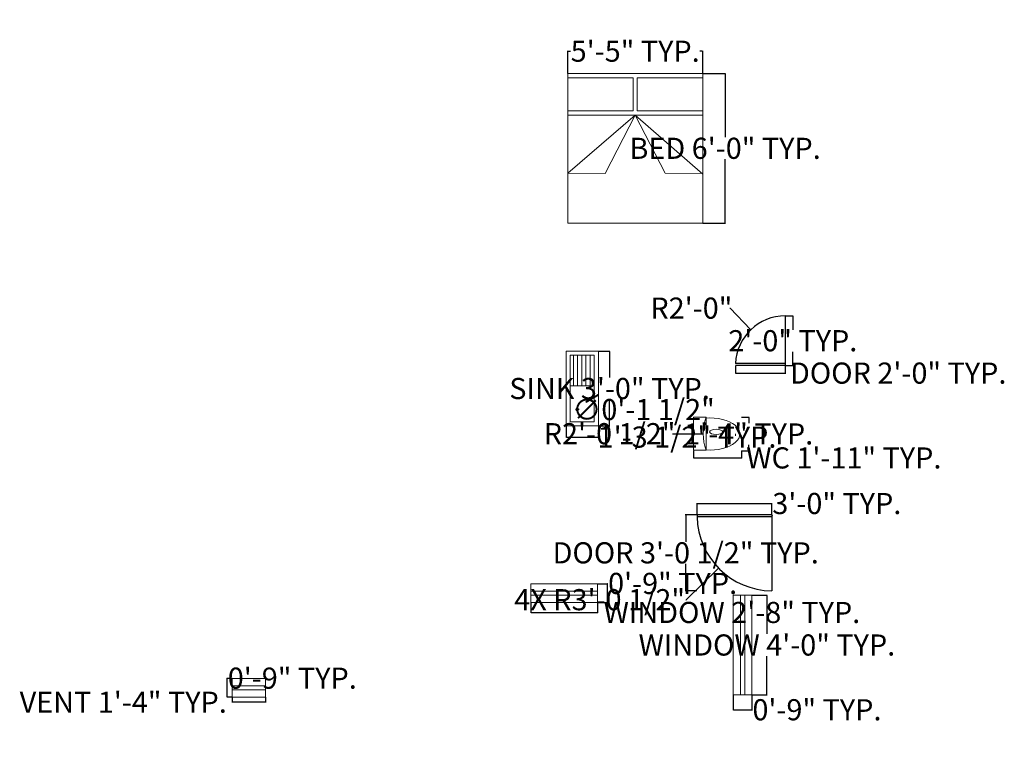
# Model space of a CAD drawing. Units: inches. Extents: x 254 to 1358, y 67 to 796.
# Tile 3 of 3: x 884 to 1358, y 443 to 796. Entities that reach past the tile are written whole.
import ezdxf

# ---------------------------------------------------------------- set-up
doc = ezdxf.new("R2010")
doc.units = ezdxf.units.IN
doc.header["$MEASUREMENT"] = 0
for name, color, linetype, lineweight in [('A-ANNO-DIMS', 2, 'Continuous', 18), ('A-FLOR-FIXT', 9, 'Continuous', 18), ('A-FURN', 8, 'Continuous', 18), ('A-GLAZ', 160, 'Continuous', 18), ('doors', 8, 'Continuous', 25)]:
    doc.layers.add(name, color=color, linetype=linetype, lineweight=lineweight)
doc.styles.get("Standard").update_dxf_attribs({"font": 'arial.ttf'})
doc.dimstyles.get("Standard").update_dxf_attribs({"dimtxt": 10.18, "dimasz": 0.18, "dimexe": 0.18, "dimexo": 0.0625, "dimgap": 0.09, "dimtad": 0, "dimtih": 1, "dimtoh": 1, "dimdec": 0, "dimzin": 0, "dimdsep": 46, "dimlunit": 3, "dimtxsty": 'Standard', "dimcen": 0.09, "dimadec": 0, "dimazin": 0, "dimtfac": 1, "dimtdec": 0, "dimtofl": 0, "dimtmove": 0, "dimatfit": 3, "dimfxl": 1, "dimtolj": 1, "dimtzin": 0, "dimarcsym": 0})

# ---------------------------------------------------------------- blocks, each defined once
blk = doc.blocks.new('WIN-48')
for p, q in [((9, 48), (0, 48)), ((0, 48), (0, 0)), ((3.5, 48), (3.5, 0)), ((5.5, 48), (5.5, 0)), ((5.5, 48), (5.5, 0)), ((5.5, 48), (5.5, 0)), ((5.5, 48), (5.5, 0)), ((9, 48), (9, 0)), ((9, 0), (0, 0))]:
    blk.add_line(p, q)
blk = doc.blocks.new('VENT-16')
for p, q in [((9, 16), (0, 16)), ((0, 16), (0, 0)), ((3.5, 16), (3.5, 0)), ((5.5, 16), (5.5, 0)), ((9, 16), (9, 0)), ((9, 0), (0, 0))]:
    blk.add_line(p, q)
blk = doc.blocks.new('WIN-32')
for p, q in [((0, 0), (0, 9)), ((32.11, 9), (0, 9)), ((32.11, 5.5), (0, 5.5)), ((32.11, 0), (32.11, 9)), ((32.11, 3.5), (0, 3.5)), ((32.11, 3.5), (0, 3.5)), ((32.11, 3.5), (0, 3.5)), ((32.11, 3.5), (0, 3.5)), ((32.11, 0), (0, 0))]:
    blk.add_line(p, q)
blk = doc.blocks.new('DOOR-SWING-36')
for p, q in [((0, 0), (-36, 0)), ((-36, 0), (-36, -1)), ((0, 0), (0, -36.57)), ((0, -1), (-36, -1))]:
    blk.add_line(p, q)
blk.add_arc((0.31, -0.26), 36.31, 181.1696, 269.5155)
blk = doc.blocks.new('DOOR-SWING-24-BATH')
for p, q in [((0, 24), (0, 0)), ((0, 1), (-24, 1)), ((0, 0), (-24, 0))]:
    blk.add_line(p, q)
blk.add_arc((0, 0), 24, 90, 177.6141)
blk = doc.blocks.new('BED-DOUBLE')
for p, q in [((65, 72), (0, 72)), ((0, 72), (0, 0)), ((65, 0), (65, 72)), ((0, 48.04), (18, 48.19)), ((32.5, 20), (0, 48.04)), ((32.5, 20), (18, 48.19)), ((32.5, 20), (65, 48.44)), ((47, 48.04), (32.5, 20)), ((47, 48.04), (65, 48.19)), ((0, 20), (65, 20)), ((0, 18), (31.5, 18)), ((31.5, 18), (31.5, 2)), ((33.5, 18), (33.5, 2)), ((33.5, 18), (65, 18)), ((0, 2), (31.5, 2)), ((0, 0), (65, 0)), ((33.5, 2), (65, 2))]:
    blk.add_line(p, q)
blk = doc.blocks.new('WC-TANK')
for p, q in [((0, 8), (0, -8)), ((0, 8), (6, 8)), ((6, 8), (6, -8)), ((20.2, -1.04), (20.22, -0.04)), ((0, -8), (6, -8))]:
    blk.add_line(p, q)
blk.add_arc((29.23, 0), 24.57, 160.9964, 199.0036)
blk.add_ellipse((7.89, -0.16), major_axis=(14.43, 0), ratio=0.535102, start_param=4.576661, end_param=7.997223)
blk.add_ellipse((10.89, 0.89), major_axis=(3.17, 0), ratio=0.394417)
blk = doc.blocks.new('SINK-DRAINBOARD')
for p, q in [((15.54, 36), (0, 36)), ((0, 36), (0, 0)), ((13.54, 34), (2, 34)), ((2, 34), (2, 2)), ((3.54, 19.32), (3.54, 34)), ((5.54, 19.32), (5.54, 34)), ((7.54, 19.32), (7.54, 34)), ((9.54, 19.32), (9.54, 34)), ((11.54, 19.32), (11.54, 34)), ((13.54, 2), (13.54, 34)), ((15.54, 0), (15.54, 36)), ((13.54, 19.32), (2, 19.32)), ((15.54, 15.32), (9.48, 11.67)), ((9.73, 11.27), (15.54, 14.86)), ((9.48, 11.67), (9.73, 11.27)), ((11.54, 12.39), (11.54, 12.92)), ((0, 0), (15.54, 0)), ((2, 2), (13.54, 2))]:
    blk.add_line(p, q)
blk.add_circle((5.29, 7.86), 0.652)
blk = doc.blocks.new('*D16')
at = {"layer": 'A-ANNO-DIMS', "color": 0, "lineweight": -2, "transparency": 16777216}
for p, q in [((1236.63, 518.72), (1243.95, 518.72)), ((1243.77, 518.54), (1243.77, 500.07)), ((1243.77, 470.9), (1243.77, 489.36)), ((1236.63, 470.72), (1243.95, 470.72))]:
    blk.add_line(p, q, dxfattribs=at)
at = {"layer": 'A-ANNO-DIMS', "color": 0, "transparency": 16777216}
for points in [[(1243.74, 518.54), (1243.8, 518.54), (1243.77, 518.72)], [(1243.74, 470.9), (1243.8, 470.9), (1243.77, 470.72)]]:
    blk.add_solid(points, dxfattribs=at)
at = {"layer": 'Defpoints', "color": 0, "transparency": 16777216}
for p in [(1236.57, 518.72), (1243.77, 518.72), (1236.57, 470.72)]:
    blk.add_point(p, dxfattribs=at)
at = {"layer": 'A-ANNO-DIMS', "color": 0, "transparency": 16777216, "insert": (1243.77, 494.72), "char_height": 10.18, "attachment_point": 5}
blk.add_mtext('\\A1;WINDOW 4\'-0" TYP.', dxfattribs=at)
blk = doc.blocks.new('*D17')
at = {"layer": 'A-ANNO-DIMS', "color": 0, "lineweight": -2, "transparency": 16777216}
for p, q in [((1227.57, 470.65), (1227.57, 463.34)), ((1236.57, 470.65), (1236.57, 463.34)), ((1227.75, 463.52), (1236.39, 463.52)), ((1236.57, 463.52), (1236.75, 463.52))]:
    blk.add_line(p, q, dxfattribs=at)
at = {"layer": 'A-ANNO-DIMS', "color": 0, "transparency": 16777216}
for points in [[(1227.75, 463.55), (1227.75, 463.49), (1227.57, 463.52)], [(1236.39, 463.55), (1236.39, 463.49), (1236.57, 463.52)]]:
    blk.add_solid(points, dxfattribs=at)
at = {"layer": 'Defpoints', "color": 0, "transparency": 16777216}
for p in [(1227.57, 470.72), (1236.57, 470.72), (1236.57, 463.52)]:
    blk.add_point(p, dxfattribs=at)
at = {"layer": 'A-ANNO-DIMS', "color": 0, "transparency": 16777216, "insert": (1267.86, 463.52), "char_height": 10.18, "attachment_point": 5}
blk.add_mtext('\\A1;0\'-9" TYP.', dxfattribs=at)
blk = doc.blocks.new('*D18')
at = {"layer": 'A-ANNO-DIMS', "color": 0, "lineweight": -2, "transparency": 16777216}
for p, q in [((1210.08, 557.42), (1204.48, 557.42)), ((1204.66, 557.24), (1204.66, 544.49)), ((1204.66, 521.03), (1204.66, 533.77)), ((1210.08, 520.85), (1204.48, 520.85))]:
    blk.add_line(p, q, dxfattribs=at)
at = {"layer": 'A-ANNO-DIMS', "color": 0, "transparency": 16777216}
for points in [[(1204.63, 557.24), (1204.69, 557.24), (1204.66, 557.42)], [(1204.63, 521.03), (1204.69, 521.03), (1204.66, 520.85)]]:
    blk.add_solid(points, dxfattribs=at)
at = {"layer": 'Defpoints', "color": 0, "transparency": 16777216}
for p in [(1204.66, 557.42), (1210.15, 557.42), (1210.15, 520.85)]:
    blk.add_point(p, dxfattribs=at)
at = {"layer": 'A-ANNO-DIMS', "color": 0, "transparency": 16777216, "insert": (1204.66, 539.13), "char_height": 10.18, "attachment_point": 5}
blk.add_mtext('\\A1;DOOR 3\'-0 1/2" TYP.', dxfattribs=at)
blk = doc.blocks.new('*D19')
at = {"layer": 'A-ANNO-DIMS', "color": 0, "lineweight": -2, "transparency": 16777216}
for p, q in [((1210.15, 557.48), (1210.15, 563.09)), ((1210.33, 562.91), (1245.97, 562.91)), ((1246.15, 557.48), (1246.15, 563.09)), ((1246.15, 562.91), (1246.33, 562.91))]:
    blk.add_line(p, q, dxfattribs=at)
at = {"layer": 'A-ANNO-DIMS', "color": 0, "transparency": 16777216}
for points in [[(1210.33, 562.94), (1210.33, 562.88), (1210.15, 562.91)], [(1245.97, 562.94), (1245.97, 562.88), (1246.15, 562.91)]]:
    blk.add_solid(points, dxfattribs=at)
at = {"layer": 'Defpoints', "color": 0, "transparency": 16777216}
for p in [(1246.15, 562.91), (1210.15, 557.42), (1246.15, 557.42)]:
    blk.add_point(p, dxfattribs=at)
at = {"layer": 'A-ANNO-DIMS', "color": 0, "transparency": 16777216, "insert": (1277.44, 562.91), "char_height": 10.18, "attachment_point": 5}
blk.add_mtext('\\A1;3\'-0" TYP.', dxfattribs=at)
blk = doc.blocks.new('*D20')
at = {"layer": 'A-ANNO-DIMS', "color": 0, "lineweight": -2, "transparency": 16777216}
for p, q in [((986.3, 469.5), (986.3, 466.98)), ((1002.3, 469.5), (1002.3, 466.98)), ((986.3, 467.16), (986.12, 467.16)), ((1002.12, 467.16), (986.48, 467.16))]:
    blk.add_line(p, q, dxfattribs=at)
at = {"layer": 'A-ANNO-DIMS', "color": 0, "transparency": 16777216}
for points in [[(986.48, 467.19), (986.48, 467.13), (986.3, 467.16)], [(1002.12, 467.19), (1002.12, 467.13), (1002.3, 467.16)]]:
    blk.add_solid(points, dxfattribs=at)
at = {"layer": 'Defpoints', "color": 0, "transparency": 16777216}
for p in [(986.3, 469.56), (1002.3, 469.56), (986.3, 467.16)]:
    blk.add_point(p, dxfattribs=at)
at = {"layer": 'A-ANNO-DIMS', "color": 0, "transparency": 16777216, "insert": (933.8, 467.16), "char_height": 10.18, "attachment_point": 5}
blk.add_mtext('\\A1;VENT 1\'-4" TYP.', dxfattribs=at)
blk = doc.blocks.new('*D21')
at = {"layer": 'A-ANNO-DIMS', "color": 0, "lineweight": -2, "transparency": 16777216}
for p, q in [((986.24, 478.56), (983.72, 478.56)), ((983.9, 478.56), (983.9, 478.74)), ((983.9, 478.74), (984.08, 478.74)), ((983.9, 469.74), (983.9, 478.38)), ((986.24, 469.56), (983.72, 469.56))]:
    blk.add_line(p, q, dxfattribs=at)
at = {"layer": 'A-ANNO-DIMS', "color": 0, "transparency": 16777216}
for points in [[(983.87, 478.38), (983.93, 478.38), (983.9, 478.56)], [(983.87, 469.74), (983.93, 469.74), (983.9, 469.56)]]:
    blk.add_solid(points, dxfattribs=at)
at = {"layer": 'Defpoints', "color": 0, "transparency": 16777216}
for p in [(983.9, 478.56), (986.3, 478.56), (986.3, 469.56)]:
    blk.add_point(p, dxfattribs=at)
at = {"layer": 'A-ANNO-DIMS', "color": 0, "transparency": 16777216, "insert": (1015.2, 478.74), "char_height": 10.18, "attachment_point": 5}
blk.add_mtext('\\A1;0\'-9" TYP.', dxfattribs=at)
blk = doc.blocks.new('*D22')
at = {"layer": 'A-ANNO-DIMS', "color": 0, "lineweight": -2, "transparency": 16777216}
for p, q in [((1212.9, 770.08), (1223.82, 770.08)), ((1223.64, 769.9), (1223.64, 739.37)), ((1223.64, 698.26), (1223.64, 728.79)), ((1212.9, 698.08), (1223.82, 698.08))]:
    blk.add_line(p, q, dxfattribs=at)
at = {"layer": 'A-ANNO-DIMS', "color": 0, "transparency": 16777216}
for points in [[(1223.61, 769.9), (1223.67, 769.9), (1223.64, 770.08)], [(1223.61, 698.26), (1223.67, 698.26), (1223.64, 698.08)]]:
    blk.add_solid(points, dxfattribs=at)
at = {"layer": 'Defpoints', "color": 0, "transparency": 16777216}
for p in [(1212.84, 770.08), (1212.84, 698.08), (1223.64, 698.08)]:
    blk.add_point(p, dxfattribs=at)
at = {"layer": 'A-ANNO-DIMS', "color": 0, "transparency": 16777216, "insert": (1223.64, 734.08), "char_height": 10.18, "attachment_point": 5}
blk.add_mtext('\\A1;BED 6\'-0" TYP.', dxfattribs=at)
blk = doc.blocks.new('*D23')
at = {"layer": 'A-ANNO-DIMS', "color": 0, "lineweight": -2, "transparency": 16777216}
for p, q in [((1147.84, 770.14), (1147.84, 781.06)), ((1148.02, 780.88), (1149.22, 780.88)), ((1212.66, 780.88), (1211.45, 780.88)), ((1212.84, 770.14), (1212.84, 781.06))]:
    blk.add_line(p, q, dxfattribs=at)
at = {"layer": 'A-ANNO-DIMS', "color": 0, "transparency": 16777216}
for points in [[(1148.02, 780.91), (1148.02, 780.85), (1147.84, 780.88)], [(1212.66, 780.91), (1212.66, 780.85), (1212.84, 780.88)]]:
    blk.add_solid(points, dxfattribs=at)
at = {"layer": 'Defpoints', "color": 0, "transparency": 16777216}
for p in [(1212.84, 780.88), (1147.84, 770.08), (1212.84, 770.08)]:
    blk.add_point(p, dxfattribs=at)
at = {"layer": 'A-ANNO-DIMS', "color": 0, "transparency": 16777216, "insert": (1180.34, 780.88), "char_height": 10.18, "attachment_point": 5}
blk.add_mtext('\\A1;5\'-5" TYP.', dxfattribs=at)
blk = doc.blocks.new('*D24')
at = {"layer": 'A-ANNO-DIMS', "color": 0, "lineweight": -2, "transparency": 16777216}
for p, q in [((1130.13, 515.16), (1130.13, 510.22)), ((1162.24, 515.16), (1162.24, 510.22)), ((1130.31, 510.4), (1162.06, 510.4)), ((1162.24, 510.4), (1162.42, 510.4))]:
    blk.add_line(p, q, dxfattribs=at)
at = {"layer": 'A-ANNO-DIMS', "color": 0, "transparency": 16777216}
for points in [[(1130.31, 510.43), (1130.31, 510.37), (1130.13, 510.4)], [(1162.06, 510.43), (1162.06, 510.37), (1162.24, 510.4)]]:
    blk.add_solid(points, dxfattribs=at)
at = {"layer": 'Defpoints', "color": 0, "transparency": 16777216}
for p in [(1130.13, 515.22), (1162.24, 515.22), (1162.24, 510.4)]:
    blk.add_point(p, dxfattribs=at)
at = {"layer": 'A-ANNO-DIMS', "color": 0, "transparency": 16777216, "insert": (1226.92, 510.4), "char_height": 10.18, "attachment_point": 5}
blk.add_mtext('\\A1;WINDOW 2\'-8" TYP.', dxfattribs=at)
blk = doc.blocks.new('*D25')
at = {"layer": 'A-ANNO-DIMS', "color": 0, "lineweight": -2, "transparency": 16777216}
for p, q in [((1162.3, 524.22), (1167.24, 524.22)), ((1167.06, 524.22), (1167.06, 524.4)), ((1167.06, 524.4), (1167.24, 524.4)), ((1167.06, 515.4), (1167.06, 524.04)), ((1162.3, 515.22), (1167.24, 515.22))]:
    blk.add_line(p, q, dxfattribs=at)
at = {"layer": 'A-ANNO-DIMS', "color": 0, "transparency": 16777216}
for points in [[(1167.03, 524.04), (1167.09, 524.04), (1167.06, 524.22)], [(1167.03, 515.4), (1167.09, 515.4), (1167.06, 515.22)]]:
    blk.add_solid(points, dxfattribs=at)
at = {"layer": 'Defpoints', "color": 0, "transparency": 16777216}
for p in [(1162.24, 524.22), (1167.06, 524.22), (1162.24, 515.22)]:
    blk.add_point(p, dxfattribs=at)
at = {"layer": 'A-ANNO-DIMS', "color": 0, "transparency": 16777216, "insert": (1198.35, 524.4), "char_height": 10.18, "attachment_point": 5}
blk.add_mtext('\\A1;0\'-9" TYP.', dxfattribs=at)
blk = doc.blocks.new('*D26')
at = {"layer": 'A-ANNO-DIMS', "color": 0, "lineweight": -2, "transparency": 16777216}
for p, q in [((1228.64, 629.29), (1228.64, 625.57)), ((1252.64, 629.29), (1252.64, 625.57)), ((1228.82, 625.75), (1252.46, 625.75)), ((1252.64, 625.75), (1252.82, 625.75))]:
    blk.add_line(p, q, dxfattribs=at)
at = {"layer": 'A-ANNO-DIMS', "color": 0, "transparency": 16777216}
for points in [[(1228.82, 625.78), (1228.82, 625.72), (1228.64, 625.75)], [(1252.46, 625.78), (1252.46, 625.72), (1252.64, 625.75)]]:
    blk.add_solid(points, dxfattribs=at)
at = {"layer": 'Defpoints', "color": 0, "transparency": 16777216}
for p in [(1228.64, 629.35), (1252.64, 629.35), (1252.64, 625.75)]:
    blk.add_point(p, dxfattribs=at)
at = {"layer": 'A-ANNO-DIMS', "color": 0, "transparency": 16777216, "insert": (1306.99, 625.75), "char_height": 10.18, "attachment_point": 5}
blk.add_mtext('\\A1;DOOR 2\'-0" TYP.', dxfattribs=at)
blk = doc.blocks.new('*D27')
at = {"layer": 'A-ANNO-DIMS', "color": 0, "lineweight": -2, "transparency": 16777216}
for p, q in [((1252.7, 653.35), (1256.42, 653.35)), ((1256.24, 653.17), (1256.24, 646.64)), ((1256.24, 629.53), (1256.24, 636.06)), ((1252.7, 629.35), (1256.42, 629.35))]:
    blk.add_line(p, q, dxfattribs=at)
at = {"layer": 'A-ANNO-DIMS', "color": 0, "transparency": 16777216}
for points in [[(1256.21, 653.17), (1256.27, 653.17), (1256.24, 653.35)], [(1256.21, 629.53), (1256.27, 629.53), (1256.24, 629.35)]]:
    blk.add_solid(points, dxfattribs=at)
at = {"layer": 'Defpoints', "color": 0, "transparency": 16777216}
for p in [(1252.64, 653.35), (1256.24, 653.35), (1252.64, 629.35)]:
    blk.add_point(p, dxfattribs=at)
at = {"layer": 'A-ANNO-DIMS', "color": 0, "transparency": 16777216, "insert": (1256.24, 641.35), "char_height": 10.18, "attachment_point": 5}
blk.add_mtext('\\A1;2\'-0" TYP.', dxfattribs=at)
blk = doc.blocks.new('*D30')
at = {"layer": 'A-ANNO-DIMS', "color": 0, "lineweight": -2, "transparency": 16777216}
for p, q in [((1208.44, 588.27), (1208.44, 584.69)), ((1231.53, 588.27), (1231.53, 584.69)), ((1208.62, 584.87), (1231.35, 584.87)), ((1231.53, 584.87), (1231.71, 584.87))]:
    blk.add_line(p, q, dxfattribs=at)
at = {"layer": 'A-ANNO-DIMS', "color": 0, "transparency": 16777216}
for points in [[(1208.62, 584.9), (1208.62, 584.84), (1208.44, 584.87)], [(1231.35, 584.9), (1231.35, 584.84), (1231.53, 584.87)]]:
    blk.add_solid(points, dxfattribs=at)
at = {"layer": 'Defpoints', "color": 0, "transparency": 16777216}
for p in [(1208.44, 588.33), (1231.53, 588.33), (1231.53, 584.87)]:
    blk.add_point(p, dxfattribs=at)
at = {"layer": 'A-ANNO-DIMS', "color": 0, "transparency": 16777216, "insert": (1280.81, 584.87), "char_height": 10.18, "attachment_point": 5}
blk.add_mtext('\\A1;WC 1\'-11" TYP.', dxfattribs=at)
blk = doc.blocks.new('*D31')
at = {"layer": 'A-ANNO-DIMS', "color": 0, "lineweight": -2, "transparency": 16777216}
for p, q in [((1231.59, 604.55), (1235.18, 604.55)), ((1235, 604.37), (1235, 601.65)), ((1231.59, 588.33), (1235.18, 588.33)), ((1235, 588.51), (1235, 591.24))]:
    blk.add_line(p, q, dxfattribs=at)
at = {"layer": 'A-ANNO-DIMS', "color": 0, "transparency": 16777216}
for points in [[(1234.97, 604.37), (1235.03, 604.37), (1235, 604.55)], [(1234.97, 588.51), (1235.03, 588.51), (1235, 588.33)]]:
    blk.add_solid(points, dxfattribs=at)
at = {"layer": 'Defpoints', "color": 0, "transparency": 16777216}
for p in [(1231.53, 604.55), (1235, 604.55), (1231.53, 588.33)]:
    blk.add_point(p, dxfattribs=at)
at = {"layer": 'A-ANNO-DIMS', "color": 0, "transparency": 16777216, "insert": (1235, 596.44), "char_height": 10.18, "attachment_point": 5}
blk.add_mtext('\\A1;1\'-4" TYP.', dxfattribs=at)
blk = doc.blocks.new('*D32')
at = {"layer": 'A-ANNO-DIMS', "color": 0, "lineweight": -2, "transparency": 16777216}
for p, q in [((1162.67, 636.31), (1168.19, 636.31)), ((1168.01, 636.13), (1168.01, 623.67)), ((1168.01, 600.49), (1168.01, 612.95)), ((1162.67, 600.31), (1168.19, 600.31))]:
    blk.add_line(p, q, dxfattribs=at)
at = {"layer": 'A-ANNO-DIMS', "color": 0, "transparency": 16777216}
for points in [[(1167.98, 636.13), (1168.04, 636.13), (1168.01, 636.31)], [(1167.98, 600.49), (1168.04, 600.49), (1168.01, 600.31)]]:
    blk.add_solid(points, dxfattribs=at)
at = {"layer": 'Defpoints', "color": 0, "transparency": 16777216}
for p in [(1162.61, 636.31), (1168.01, 636.31), (1162.61, 600.31)]:
    blk.add_point(p, dxfattribs=at)
at = {"layer": 'A-ANNO-DIMS', "color": 0, "transparency": 16777216, "insert": (1168.01, 618.31), "char_height": 10.18, "attachment_point": 5}
blk.add_mtext('\\A1;SINK 3\'-0" TYP.', dxfattribs=at)
blk = doc.blocks.new('*D33')
at = {"layer": 'A-ANNO-DIMS', "color": 0, "lineweight": -2, "transparency": 16777216}
for p, q in [((1147.07, 600.25), (1147.07, 594.73)), ((1162.61, 600.25), (1162.61, 594.73)), ((1147.25, 594.91), (1162.43, 594.91)), ((1162.61, 594.91), (1162.79, 594.91))]:
    blk.add_line(p, q, dxfattribs=at)
at = {"layer": 'A-ANNO-DIMS', "color": 0, "transparency": 16777216}
for points in [[(1147.25, 594.94), (1147.25, 594.88), (1147.07, 594.91)], [(1162.43, 594.94), (1162.43, 594.88), (1162.61, 594.91)]]:
    blk.add_solid(points, dxfattribs=at)
at = {"layer": 'Defpoints', "color": 0, "transparency": 16777216}
for p in [(1147.07, 600.31), (1162.61, 600.31), (1162.61, 594.91)]:
    blk.add_point(p, dxfattribs=at)
at = {"layer": 'A-ANNO-DIMS', "color": 0, "transparency": 16777216, "insert": (1205.29, 594.91), "char_height": 10.18, "attachment_point": 5}
blk.add_mtext('\\A1;1\'-3 1/2" TYP.', dxfattribs=at)
blk = doc.blocks.new('*D57')
at = {"layer": 'A-ANNO-DIMS', "color": 0, "lineweight": -2, "transparency": 16777216}
for p, q in [((1246.36, 557.16), (1246.54, 557.16)), ((1246.45, 557.07), (1246.45, 557.25)), ((1204.89, 516.55), (1220.35, 531.66)), ((1204.71, 516.55), (1204.89, 516.55))]:
    blk.add_line(p, q, dxfattribs=at)
at = {"layer": 'A-ANNO-DIMS', "color": 0, "transparency": 16777216}
blk.add_solid([(1220.33, 531.68), (1220.37, 531.63), (1220.48, 531.78)], dxfattribs=at)
at = {"layer": 'Defpoints', "color": 0, "transparency": 16777216}
for p in [(1246.45, 557.16), (1220.48, 531.78)]:
    blk.add_point(p, dxfattribs=at)
at = {"layer": 'A-ANNO-DIMS', "color": 0, "transparency": 16777216, "insert": (1163.22, 516.55), "char_height": 10.18, "attachment_point": 5}
blk.add_mtext('\\A1;4X R3\'-0 1/2"', dxfattribs=at)
blk = doc.blocks.new('*D58')
at = {"layer": 'A-ANNO-DIMS', "color": 0, "lineweight": -2, "transparency": 16777216}
for p, q in [((1225.88, 657.06), (1226.06, 657.06)), ((1226.06, 657.06), (1235.9, 646.8)), ((1252.55, 629.35), (1252.73, 629.35)), ((1252.64, 629.26), (1252.64, 629.44))]:
    blk.add_line(p, q, dxfattribs=at)
at = {"layer": 'A-ANNO-DIMS', "color": 0, "transparency": 16777216}
blk.add_solid([(1235.93, 646.82), (1235.88, 646.78), (1236.03, 646.67)], dxfattribs=at)
at = {"layer": 'Defpoints', "color": 0, "transparency": 16777216}
for p in [(1236.03, 646.67), (1252.64, 629.35)]:
    blk.add_point(p, dxfattribs=at)
at = {"layer": 'A-ANNO-DIMS', "color": 0, "transparency": 16777216, "insert": (1207.39, 657.06), "char_height": 10.18, "attachment_point": 5}
blk.add_mtext('\\A1;R2\'-0"', dxfattribs=at)
blk = doc.blocks.new('*D60')
at = {"layer": 'A-ANNO-DIMS', "color": 0, "lineweight": -2, "transparency": 16777216}
for p, q in [((1198.36, 596.55), (1212.92, 596.55)), ((1237.58, 596.55), (1237.76, 596.55)), ((1237.67, 596.46), (1237.67, 596.64))]:
    blk.add_line(p, q, dxfattribs=at)
at = {"layer": 'A-ANNO-DIMS', "color": 0, "transparency": 16777216}
blk.add_solid([(1212.92, 596.58), (1212.92, 596.52), (1213.1, 596.55)], dxfattribs=at)
at = {"layer": 'Defpoints', "color": 0, "transparency": 16777216}
for p in [(1213.1, 596.55), (1237.67, 596.55)]:
    blk.add_point(p, dxfattribs=at)
at = {"layer": 'A-ANNO-DIMS', "color": 0, "transparency": 16777216, "insert": (1168.01, 596.55), "char_height": 10.18, "attachment_point": 5}
blk.add_mtext('\\A1;R2\'-0 1/2"', dxfattribs=at)
blk = doc.blocks.new('*D61')
at = {"layer": 'A-ANNO-DIMS', "color": 0, "lineweight": -2, "transparency": 16777216}
for p, q in [((1152.26, 608.17), (1152.44, 608.17)), ((1152.35, 608.08), (1152.35, 608.26)), ((1153.4, 608.17), (1153.18, 608.17))]:
    blk.add_line(p, q, dxfattribs=at)
at = {"layer": 'A-ANNO-DIMS', "color": 0, "transparency": 16777216}
blk.add_solid([(1153.18, 608.2), (1153.18, 608.14), (1153, 608.17)], dxfattribs=at)
at = {"layer": 'Defpoints', "color": 0, "transparency": 16777216}
for p in [(1151.7, 608.17), (1153, 608.17)]:
    blk.add_point(p, dxfattribs=at)
at = {"layer": 'A-ANNO-DIMS', "color": 0, "transparency": 16777216, "insert": (1184.41, 608.17), "char_height": 10.18, "attachment_point": 5}
blk.add_mtext('\\A1;∅0\'-1 1/2"', dxfattribs=at)

msp = doc.modelspace()

# ---------------------------------------------------------------- block references
at = {"layer": 'A-FLOR-FIXT'}
for name, p in [('SINK-DRAINBOARD', (1147.07, 600.31)), ('WC-TANK', (1208.44, 596.55))]:
    msp.add_blockref(name, p, dxfattribs=at)
at = {"layer": 'A-FURN', "extrusion": (0, 0, -1), "zscale": -1, "rotation": 180}
msp.add_blockref('BED-DOUBLE', (-1147.84, 770.08), dxfattribs=at)
at = {"layer": 'A-GLAZ'}
for name, p in [('WIN-32', (1130.13, 515.22)), ('WIN-48', (1227.57, 470.72))]:
    msp.add_blockref(name, p, dxfattribs=at)
at = {"layer": 'A-GLAZ', "rotation": 89.99999999999844}
msp.add_blockref('VENT-16', (1002.3, 469.56), dxfattribs=at)
at = {"layer": 'doors'}
for name, p in [('DOOR-SWING-24-BATH', (1252.64, 629.35)), ('DOOR-SWING-36', (1246.15, 557.42))]:
    msp.add_blockref(name, p, dxfattribs=at)

# ---------------------------------------------------------------- dimensions: what is measured, and where the dimension line sits
at = {"layer": 'A-ANNO-DIMS'}
for base, p1, p2, text, picture, middle in [((1212.84, 780.88), (1147.84, 770.08), (1212.84, 770.08), '<> TYP.', '*D23', (1180.34, 780.88)), ((1252.64, 625.75), (1228.64, 629.35), (1252.64, 629.35), 'DOOR <> TYP.', '*D26', (1306.99, 625.75)), ((1162.61, 594.91), (1147.07, 600.31), (1162.61, 600.31), '<> TYP.', '*D33', (1205.29, 594.91)), ((1231.53, 584.87), (1208.44, 588.33), (1231.53, 588.33), 'WC <> TYP.', '*D30', (1280.81, 584.87)), ((1246.15, 562.91), (1210.15, 557.42), (1246.15, 557.42), '<> TYP.', '*D19', (1277.44, 562.91)), ((1162.24, 510.4), (1130.13, 515.22), (1162.24, 515.22), 'WINDOW <> TYP.', '*D24', (1226.92, 510.4)), ((1236.57, 463.52), (1227.57, 470.72), (1236.57, 470.72), '<> TYP.', '*D17', (1267.86, 463.52))]:
    dim = msp.add_linear_dim(base=base, p1=p1, p2=p2, text=text, dimstyle='Standard', override={"dimdec": 1, "dimlfac": 1, "dimrnd": 0, "dimzin": 1, "dimdsep": 46, "dimlunit": 4, "dimfrac": 2}, dxfattribs=at)
    dim.commit()
    dim.dimension.update_dxf_attribs({"geometry": picture, "text_midpoint": middle})
for base, p1, p2, angle, text, picture, middle in [((1223.64, 698.08), (1212.84, 770.08), (1212.84, 698.08), 270, 'BED <> TYP.', '*D22', (1223.64, 734.08)), ((1256.24, 653.35), (1252.64, 629.35), (1252.64, 653.35), 90, '<> TYP.', '*D27', (1256.24, 641.35)), ((1168.01, 636.31), (1162.61, 600.31), (1162.61, 636.31), 90, 'SINK <> TYP.', '*D32', (1168.01, 618.31)), ((1235, 604.55), (1231.53, 588.33), (1231.53, 604.55), 90, '<> TYP.', '*D31', (1235, 596.44)), ((1204.66, 557.42), (1210.15, 520.85), (1210.15, 557.42), 90, 'DOOR <> TYP.', '*D18', (1204.66, 539.13)), ((1167.06, 524.22), (1162.24, 515.22), (1162.24, 524.22), 90, '<> TYP.', '*D25', (1198.35, 524.4)), ((1243.77, 518.72), (1236.57, 470.72), (1236.57, 518.72), 90, 'WINDOW <> TYP.', '*D16', (1243.77, 494.72)), ((983.9, 478.56), (986.3, 469.56), (986.3, 478.56), 90, '<> TYP.', '*D21', (1015.2, 478.74)), ((986.3, 467.16), (1002.3, 469.56), (986.3, 469.56), 180, 'VENT <> TYP.', '*D20', (933.8, 467.16))]:
    dim = msp.add_linear_dim(base=base, p1=p1, p2=p2, angle=angle, text=text, dimstyle='Standard', override={"dimdec": 1, "dimlfac": 1, "dimrnd": 0, "dimzin": 1, "dimdsep": 46, "dimlunit": 4, "dimfrac": 2}, dxfattribs=at)
    dim.commit()
    dim.dimension.update_dxf_attribs({"geometry": picture, "text_midpoint": middle})
for center, mpoint, picture, middle in [((1252.64, 629.35), (1236.03, 646.67), '*D58', (1207.39, 657.06)), ((1237.67, 596.55), (1213.1, 596.55), '*D60', (1198.36, 596.55))]:
    dim = msp.add_radius_dim(center=center, mpoint=mpoint, dimstyle='Standard', override={"dimdec": 1, "dimlfac": 1, "dimrnd": 0, "dimzin": 1, "dimdsep": 46, "dimlunit": 4, "dimfrac": 2}, dxfattribs=at)
    dim.commit()
    dim.dimension.update_dxf_attribs({"geometry": picture, "text_midpoint": middle, "dimtype": 164})
dim = msp.add_diameter_dim_2p(p1=(1151.7, 608.17), p2=(1153, 608.17), dimstyle='Standard', override={"dimdec": 1, "dimlfac": 1, "dimrnd": 0, "dimzin": 1, "dimdsep": 46, "dimlunit": 4, "dimfrac": 2}, dxfattribs=at)
dim.commit()
dim.dimension.update_dxf_attribs({"geometry": '*D61', "text_midpoint": (1153.4, 608.17), "dimtype": 163})
dim = msp.add_radius_dim(center=(1246.45, 557.16), mpoint=(1220.48, 531.78), text='4X <>', dimstyle='Standard', override={"dimdec": 1, "dimlfac": 1, "dimrnd": 0, "dimzin": 1, "dimdsep": 46, "dimlunit": 4, "dimfrac": 2}, dxfattribs=at)
dim.commit()
dim.dimension.update_dxf_attribs({"geometry": '*D57', "text_midpoint": (1163.22, 516.55), "dimtype": 164})

doc.saveas('drawing.dxf')
